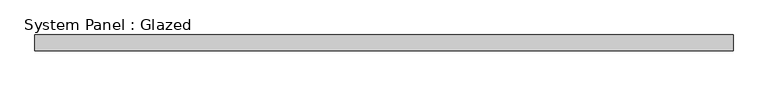
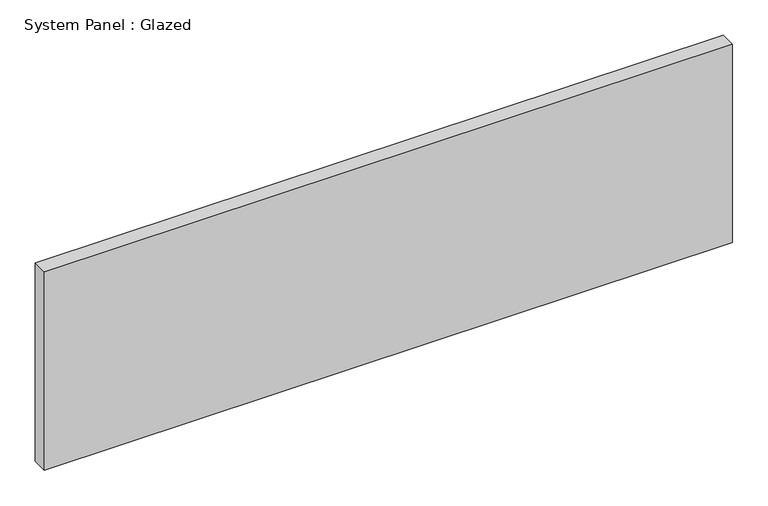
"""IFC4 building model written with IfcOpenShell, lengths in millimetres: plate geometry, System Panel : Glazed."""

from ifc_helpers import new_model, si_unit, origin, origin_with_axes, place, context, project, spatial, polyline, outline, extrude, source, transform, mapped, element, save


def system_panel_glazed_01dbb714(model_context):
    return source(origin(), model_context, "Body", "SweptSolid", [
        extrude(outline(polyline([(561.975, -44.45), (-561.975, -44.45), (-561.975, -19.05), (561.975, -19.05), (561.975, -44.45)])), origin_with_axes(), (0.0, 0.0, 1.0), 342.9),
    ])


if __name__ == "__main__":
    model = new_model("IFC4")
    model_context = context("Model", 3, world=origin())
    ifc_project = project(units=[si_unit("LENGTHUNIT", "METRE", prefix="MILLI")], contexts=[model_context])
    site = spatial("IfcSite", under=ifc_project)
    building = spatial("IfcBuilding", under=site)
    placement = place(None, origin())
    system_panel_glazed_shape = system_panel_glazed_01dbb714(model_context)
    element("IfcPlate", 1, ObjectType="System Panel : Glazed", at=placement, inside=building, context=model_context, shape_type="MappedRepresentation", body=[
        mapped(system_panel_glazed_shape, transform((0.0, 0.0, 0.0), x_axis=(1.0, 0.0, 0.0), y_axis=(0.0, 1.0, 0.0), z_axis=(0.0, 0.0, 1.0))),
    ])
    save(model, "model.ifc")

# Revit data of these elements
# Type "System Panel : Glazed"
#   Construction Type Id = "GSP4R"
#   Analytic Construction = "1/8 in Pilkington single glazing"
#   Visual Light Transmittance = 0.9
#   Solar Heat Gain Coefficient = 0.86
#   Heat Transfer Coefficient (U) = 1.18115 BTU/(h·ft²·°F)
#   Define Thermal Properties by = 1
# Element 1 (IfcPlate, "System Panel : Glazed")
#   Materials on its faces: "GARAGE PANEL"
# Materials
#   "GARAGE PANEL": class "Generic", colour RGB 120 120 120, transparency 0, Cost = 0
